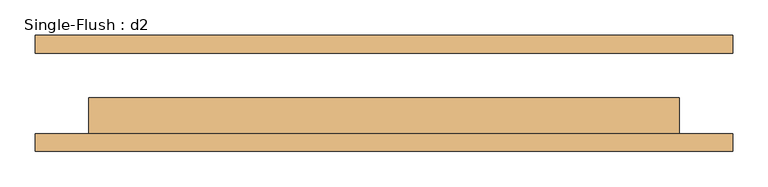
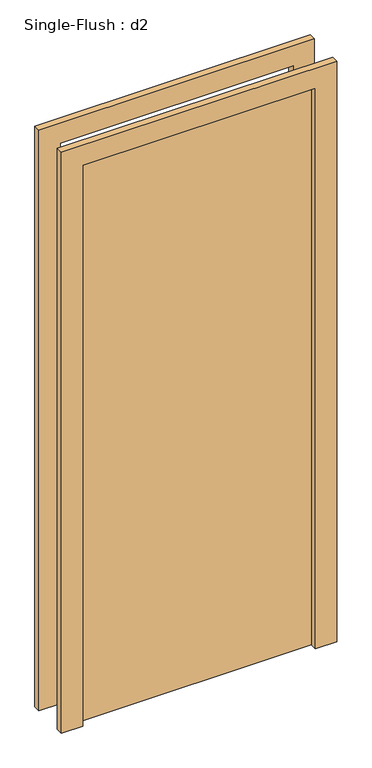
"""IFC4 building model written with IfcOpenShell, lengths in millimetres: door geometry, Single-Flush : d2."""

from ifc_helpers import new_model, si_unit, frame, origin, origin_with_axes, place, context, project, spatial, polyline, outline, extrude, source, transform, mapped, element, save


def single_flush_d2_19300210(model_context):
    return source(origin(), model_context, "Body", "SweptSolid", [
        extrude(outline(polyline([(2209.8, -495.3), (0.0, -495.3), (0.0, -419.1), (2133.6, -419.1), (2133.6, 419.1), (0.0, 419.1), (0.0, 495.3), (2209.8, 495.3), (2209.8, -495.3)])), frame((0.0, -82.55, 0.0), z_axis=(0.0, 1.0, 0.0), x_axis=(0.0, 0.0, 1.0)), (0.0, 0.0, 1.0), 25.4),
        extrude(outline(polyline([(2209.8, 495.3), (2209.8, -495.3), (0.0, -495.3), (0.0, -419.1), (2133.6, -419.1), (2133.6, 419.1), (0.0, 419.1), (0.0, 495.3), (2209.8, 495.3)])), frame((0.0, 57.15, 0.0), z_axis=(0.0, 1.0, 0.0), x_axis=(0.0, 0.0, 1.0)), (0.0, 0.0, 1.0), 25.4),
        extrude(outline(polyline([(419.1, -6.35), (419.1, -57.15), (-419.1, -57.15), (-419.1, -6.35), (419.1, -6.35)])), origin_with_axes(), (0.0, 0.0, 1.0), 2133.6),
    ])


if __name__ == "__main__":
    model = new_model("IFC4")
    model_context = context("Model", 3, world=origin())
    ifc_project = project(units=[si_unit("LENGTHUNIT", "METRE", prefix="MILLI")], contexts=[model_context])
    site = spatial("IfcSite", under=ifc_project)
    building = spatial("IfcBuilding", under=site)
    placement = place(None, origin())
    single_flush_d2_shape = single_flush_d2_19300210(model_context)
    element("IfcDoor", 1, ObjectType="Single-Flush : d2", at=placement, inside=building, context=model_context, shape_type="MappedRepresentation", body=[
        mapped(single_flush_d2_shape, transform((0.0, 0.0, 0.0), x_axis=(1.0, 0.0, 0.0), y_axis=(0.0, 1.0, 0.0), z_axis=(0.0, 0.0, 1.0))),
    ])
    save(model, "model.ifc")

# Revit data of these elements
# Type "Single-Flush : d2"
#   Type Mark = "9"
#   Construction Type Id = "MDOOR"
#   Assembly Code = "C1020"
#   Analytic Construction = "Metal"
#   Thickness = 0' - 2"
#   Heat Transfer Coefficient (U) = 0.651978 BTU/(h·ft²·°F)
#   Height = 7' - 0"
#   Trim Projection Ext = 0' - 1"
#   Trim Projection Int = 0' - 1"
#   Trim Width = 0' - 3"
#   Width = 2' - 9"
#   Define Thermal Properties by = 1
#   Door Material = Door - Panel
#   Frame Material = Door - Frame
#   Visual Light Transmittance = 0
#   Solar Heat Gain Coefficient = 0
#   Function = (empty or 0)
#   Wall Closure = (empty or 0)
# Element 1 (IfcDoor, "Single-Flush : d2")
#   Materials on its faces: "Door - Frame", "Door - Panel"
# Materials
#   "Door - Panel": class "Wood", colour RGB 210 159 95, transparency 0, Cost = 0
#   "Door - Frame": colour RGB 118 70 51, transparency 0, Cost = 0
